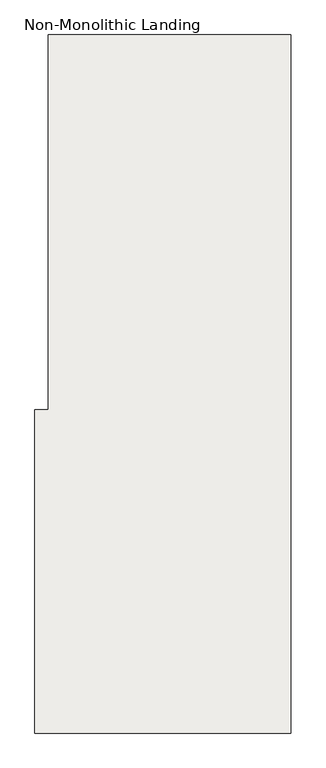
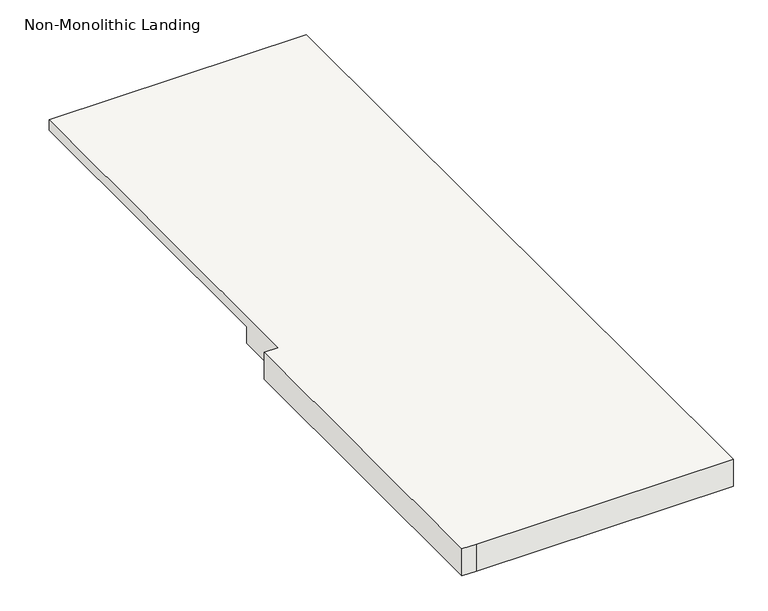
"""IFC4 building model written with IfcOpenShell, lengths in millimetres: slab geometry, Non-Monolithic Landing."""

from ifc_helpers import new_model, si_unit, origin, place, context, project, spatial, faceted_brep, source, transform, mapped, element, save


def non_monolithic_landing_3bfbdf2e(model_context):
    return source(origin(), model_context, "Body", "Brep", [
        faceted_brep([(-3732.7409298, -3238.4779636, 4781.55), (-3707.3409298, -3238.4779636, 4756.15), (-3707.3409298, -3848.0779636, 4756.15), (-3732.7409298, -3848.0779636, 4781.55), (-3732.7409298, -3945.3664375, 4800.6), (-3758.1409298, -3945.3664375, 4800.6), (-3758.1409298, -4554.9664375, 4800.6), (-3732.7409298, -4554.9664375, 4800.6), (-3275.5409298, -4554.9664375, 4800.6), (-3275.5409298, -3238.4779636, 4800.6), (-3732.7409298, -3238.4779636, 4800.6), (-3707.3409298, -3848.0779636, 4749.8), (-3707.3409298, -3238.4779636, 4749.8), (-3275.5409298, -3238.4779636, 4749.8), (-3275.5409298, -4554.9664375, 4749.8), (-3732.7409298, -4554.9664375, 4749.8), (-3758.1409298, -4554.9664375, 4749.8), (-3758.1409298, -3945.3664375, 4749.8), (-3732.7409298, -3945.3664375, 4749.8), (-3732.7409298, -3848.0779636, 4749.8)], [[[0, 1, 2, 3]], [[4, 5, 6, 7, 8, 9, 10]], [[11, 12, 13, 14, 15, 16, 17, 18, 19]], [[12, 11, 2, 1]], [[11, 19, 3, 2]], [[4, 10, 0, 3, 19, 18]], [[5, 4, 18, 17]], [[6, 5, 17, 16]], [[7, 6, 16, 15]], [[8, 7, 15, 14]], [[9, 8, 14, 13]], [[10, 9, 13, 12, 1, 0]]]),
    ])


if __name__ == "__main__":
    model = new_model("IFC4")
    model_context = context("Model", 3, world=origin())
    ifc_project = project(units=[si_unit("LENGTHUNIT", "METRE", prefix="MILLI")], contexts=[model_context])
    site = spatial("IfcSite", under=ifc_project)
    building = spatial("IfcBuilding", under=site)
    placement = place(None, origin())
    non_monolithic_landing_shape = non_monolithic_landing_3bfbdf2e(model_context)
    element("IfcSlab", 1, ObjectType="Non-Monolithic Landing", at=placement, inside=building, context=model_context, shape_type="MappedRepresentation", body=[
        mapped(non_monolithic_landing_shape, transform((0.0, 0.0, 0.0), x_axis=(1.0, 0.0, 0.0), y_axis=(0.0, 1.0, 0.0), z_axis=(0.0, 0.0, 1.0))),
    ])
    save(model, "model.ifc")
